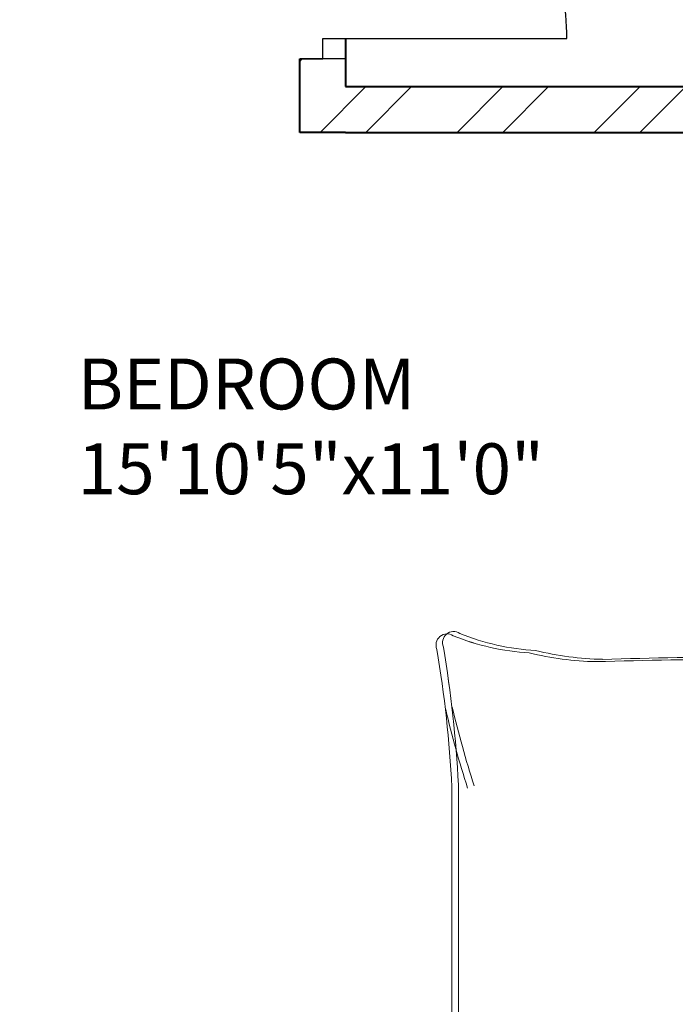
# Model space of a CAD drawing. Units: inches. Extents: x 1601 to 2297, y 1496 to 2631.
# Tile 47 of 57: x 2102 to 2167, y 2141 to 2237. Entities that reach past the tile are written whole.
import ezdxf

# ---------------------------------------------------------------- set-up
doc = ezdxf.new("R2010")
doc.units = ezdxf.units.IN
for name, color, linetype, lineweight in [('A-AREA-IDEN', 7, 'Continuous', 18), ('A-DOOR', 21, 'Continuous', 25), ('A-FURN', 8, 'Continuous', 18), ('A-WALL', 7, 'Continuous', 40), ('A-WALL-PATT', 215, 'Continuous', 13)]:
    doc.layers.add(name, color=color, linetype=linetype, lineweight=lineweight)
doc.styles.get("Standard").update_dxf_attribs({"font": 'arial.ttf'})

# ---------------------------------------------------------------- blocks, each defined once
blk = doc.blocks.new('BED-DOUBLE')
for p, q in [((79.245, 15.063), (79.245, 39.677)), ((79.245, 15.063), (79.245, 39.677)), ((79.245, 15.063), (79.245, 39.677)), ((79.245, 15.063), (79.245, 39.677)), ((79.884, 15.292), (79.884, 39.905)), ((79.884, 15.291), (79.884, 39.905)), ((79.884, 15.292), (79.884, 39.905)), ((79.884, 15.291), (79.884, 39.905))]:
    blk.add_line(p, q)
for centre, radius, start, end in [((-23.712, -17.222), 106.459, 13.38322, 17.70533), ((-23.712, -17.222), 106.459, 13.38322, 17.70533), ((-23.712, -17.222), 106.459, 13.38322, 17.70533), ((-23.712, -17.222), 106.459, 13.38322, 17.70533), ((-23.073, -16.994), 106.459, 13.38322, 17.70533), ((-23.073, -16.994), 106.459, 13.38322, 17.70533), ((-23.073, -16.994), 106.459, 13.38322, 17.70533), ((-23.073, -16.994), 106.459, 13.38322, 17.70533), ((200.837, 21.427), 121.759, 182.99578, 189.40907), ((200.837, 21.426), 121.759, 182.99578, 189.40907), ((200.837, 21.427), 121.759, 182.99578, 189.40907), ((200.837, 21.426), 121.759, 182.99578, 189.40907), ((201.476, 21.655), 121.759, 182.99578, 189.40907), ((201.476, 21.655), 121.759, 182.99578, 189.40907), ((201.476, 21.655), 121.759, 182.99578, 189.40907), ((201.476, 21.655), 121.759, 182.99578, 189.40907), ((51.253, 485.051), 482.31, 268.22771, 271.71854), ((51.253, 485.05), 482.31, 268.22771, 271.71854), ((51.253, 485.051), 482.31, 268.22771, 271.71854), ((51.253, 485.05), 482.31, 268.22771, 271.71854), ((65.154, -26.671), 29.634, 76.06484, 88.91125), ((65.154, -26.672), 29.634, 76.06484, 88.91125), ((65.154, -26.671), 29.634, 76.06484, 88.91125), ((65.154, -26.672), 29.634, 76.06484, 88.91125), ((50.614, 484.822), 482.31, 268.22771, 271.71854), ((50.614, 484.822), 482.31, 268.22771, 271.71854), ((50.614, 484.822), 482.31, 268.22771, 271.71854), ((50.614, 484.822), 482.31, 268.22771, 271.71854), ((64.515, -26.9), 29.634, 76.06484, 88.91125), ((64.515, -26.9), 29.634, 76.06484, 88.91125), ((64.515, -26.9), 29.634, 76.06484, 88.91125), ((64.515, -26.9), 29.634, 76.06484, 88.91125), ((70.915, -21.431), 23.562, 67.97508, 86.652), ((70.915, -21.432), 23.562, 67.97508, 86.652), ((70.915, -21.431), 23.562, 67.97508, 86.652), ((70.915, -21.432), 23.562, 67.97508, 86.652), ((70.276, -21.66), 23.562, 67.97508, 86.652), ((70.276, -21.66), 23.562, 67.97508, 86.652), ((70.276, -21.66), 23.562, 67.97508, 86.652), ((70.276, -21.66), 23.562, 67.97508, 86.652), ((79.718, 1.087), 1.089, 236.17358, 23.47814), ((79.718, 1.087), 1.089, 236.17358, 23.47814), ((79.718, 1.087), 1.089, 236.17358, 23.47814), ((79.718, 1.087), 1.089, 236.17358, 23.47814), ((80.357, 1.316), 1.089, 236.17358, 23.47814), ((80.357, 1.316), 1.089, 236.17358, 23.47814), ((80.357, 1.315), 1.089, 236.17358, 23.47814), ((80.357, 1.315), 1.089, 236.17358, 23.47814)]:
    blk.add_arc(centre, radius, start, end)

msp = doc.modelspace()

# ---------------------------------------------------------------- hatches: boundary and pattern name
at = {"layer": 'A-WALL-PATT'}
h = msp.add_hatch(dxfattribs=at)
h.set_pattern_fill('ANSI32', color=256)
h.paths.add_polyline_path([(1842.0336, 2528.0767), (1842.0336, 2532.3254), (1686.0373, 2532.3254), (1686.0373, 2492.9493), (1695.0373, 2492.9493), (1695.0373, 2523.3254), (1827.0373, 2523.3254), (1827.0373, 2416.8254), (1834.6225, 2416.8254), (1834.6225, 2419.0754), (1834.6225, 2421.3254), (1831.5373, 2421.3254), (1831.5373, 2523.3254), (1842.0336, 2523.3254)])
h.paths.add_polyline_path([(1695.0373, 2432.9493), (1686.0373, 2432.9493), (1686.0373, 2325.989), (1695.0373, 2325.989), (1695.0373, 2347.8254), (1827.0373, 2347.8254), (1827.0373, 2287.8254), (1823.2991, 2287.8254), (1823.2991, 2283.3254), (1847.9422, 2283.3254), (1847.9422, 2285.5754), (1847.9422, 2287.8254), (1831.5373, 2287.8254), (1831.5373, 2347.8254), (1846.9946, 2347.8254), (1846.9946, 2350.0754), (1846.9946, 2352.3254), (1695.0373, 2352.3254)])
h.paths.add_polyline_path([(1807.1169, 1573.5395), (2055.0405, 1573.5395), (2055.0405, 1610.6322), (1807.1169, 1610.6322)], flags=9)
h.paths.add_polyline_path([(1841.1631, 1712.7967), (1870.3957, 1712.7967), (1870.3957, 1731.454), (1841.1631, 1731.454)], flags=9)
h.paths.add_polyline_path([(2144.3862, 1772.185), (2191.0233, 1772.185), (2191.0233, 1790.8423), (2144.3862, 1790.8423)], flags=9)
h.paths.add_polyline_path([(2143.0128, 1827.3312), (2177.9958, 1827.3312), (2177.9958, 1845.9886), (2143.0128, 1845.9886)], flags=9)
h.paths.add_polyline_path([(2041.2439, 1833.5691), (2070.8516, 1833.5691), (2070.8516, 1852.2264), (2041.2439, 1852.2264)], flags=9)
h.paths.add_polyline_path([(2097.2791, 1947.0598), (2134.2061, 1947.0598), (2134.2061, 1965.7171), (2097.2791, 1965.7171)], flags=9)
h.paths.add_polyline_path([(2214.995, 1904.3124), (2214.995, 1942.2899), (2196.3376, 1942.2899), (2196.3376, 1904.3124)], flags=9)
h.paths.add_polyline_path([(2186.6284, 2043.8031), (2219.7935, 2043.8031), (2219.7935, 2062.4605), (2186.6284, 2062.4605)], flags=9)
h.paths.add_polyline_path([(2064.0877, 2031.616), (2097.4949, 2031.616), (2097.4949, 2050.2734), (2064.0877, 2050.2734)], flags=9)
h.paths.add_polyline_path([(1973.1349, 1986.0688), (2008.4009, 1986.0688), (2008.4009, 2004.7261), (1973.1349, 2004.7261)], flags=9)
h.paths.add_polyline_path([(1976.3676, 2106.9635), (2005.7469, 2106.9635), (2005.7469, 2125.6209), (1976.3676, 2125.6209)], flags=9)
h.paths.add_polyline_path([(1991.7852, 2180.4863), (2027.0513, 2180.4863), (2027.0513, 2199.1437), (1991.7852, 2199.1437)], flags=9)
h.paths.add_polyline_path([(2106.1801, 2187.9359), (2152.2101, 2187.9359), (2152.2101, 2206.5932), (2106.1801, 2206.5932)], flags=9)
h.paths.add_polyline_path([(2148.6686, 2262.2542), (2182.318, 2262.2542), (2182.318, 2280.9115), (2148.6686, 2280.9115)], flags=9)
h.paths.add_polyline_path([(2041.6327, 2252.8147), (2071.2405, 2252.8147), (2071.2405, 2271.4721), (2041.6327, 2271.4721)], flags=9)
h.paths.add_polyline_path([(2063.9734, 2375.4265), (2100.9004, 2375.4265), (2100.9004, 2394.0839), (2063.9734, 2394.0839)], flags=9)
h.paths.add_polyline_path([(2216.4955, 2330.9748), (2216.4955, 2370.2654), (2197.8381, 2370.2654), (2197.8381, 2330.9748)], flags=9)
h.paths.add_polyline_path([(2179.1416, 2485.8687), (2212.3067, 2485.8687), (2212.3067, 2504.5261), (2179.1416, 2504.5261)], flags=9)
h.paths.add_polyline_path([(2078.7442, 2471.1516), (2112.1514, 2471.1516), (2112.1514, 2489.809), (2078.7442, 2489.809)], flags=9)
h.paths.add_polyline_path([(1915.9631, 2329.4668), (1952.8902, 2329.4668), (1952.8902, 2348.1241), (1915.9631, 2348.1241)], flags=9)
h.paths.add_polyline_path([(1904.3189, 2499.6709), (1940.4512, 2499.6709), (1940.4512, 2518.3282), (1904.3189, 2518.3282)], flags=9)
h.paths.add_polyline_path([(1892.3665, 2100.4595), (1925.6374, 2100.4595), (1925.6374, 2119.1169), (1892.3665, 2119.1169)], flags=9)
h.paths.add_polyline_path([(1909.2984, 1805.9631), (1946.2254, 1805.9631), (1946.2254, 1824.6205), (1909.2984, 1824.6205)], flags=9)
h.paths.add_polyline_path([(1934.6056, 1658.616), (1970.738, 1658.616), (1970.738, 1677.2733), (1934.6056, 1677.2733)], flags=9)
h.paths.add_polyline_path([(1711.2052, 1789.8902), (1750.0456, 1789.8902), (1750.0456, 1808.5476), (1711.2052, 1808.5476)], flags=9)
h.paths.add_polyline_path([(1742.7874, 1854.6743), (1771.9449, 1854.6743), (1771.9449, 1873.3317), (1742.7874, 1873.3317)], flags=9)
h.paths.add_polyline_path([(1807.3592, 1997.7912), (1850.1116, 1997.7912), (1850.1116, 2016.4486), (1807.3592, 2016.4486)], flags=9)
h.paths.add_polyline_path([(1717.4579, 2237.7844), (1760.2103, 2237.7844), (1760.2103, 2256.4417), (1717.4579, 2256.4417)], flags=9)
h.paths.add_polyline_path([(1780.9285, 2324.0623), (1810.086, 2324.0623), (1810.086, 2342.7197), (1780.9285, 2342.7197)], flags=25)
h.paths.add_polyline_path([(1837.696, 2449.2024), (1866.9286, 2449.2024), (1866.9286, 2467.8598), (1837.696, 2467.8598)], flags=9)
h.paths.add_polyline_path([(1712.7752, 2484.9404), (1751.6156, 2484.9404), (1751.6156, 2503.5977), (1712.7752, 2503.5977)], flags=25)
h = msp.add_hatch(dxfattribs=at)
h.set_pattern_fill('ANSI32', color=256)
h.paths.add_polyline_path([(1973.9371, 2211.3254), (1893.0373, 2211.3254), (1893.0373, 2287.8254), (1884.6167, 2287.8254), (1884.6167, 2285.5754), (1884.6167, 2283.3254), (1888.5373, 2283.3254), (1888.5373, 2145.3254), (1695.0373, 2145.3254), (1695.0373, 2173.8724), (1690.5373, 2173.8724), (1686.0373, 2173.8724), (1686.0373, 2136.3254), (1722.5687, 2136.3254), (1722.5687, 2117.4352), (1731.5687, 2117.4352), (1731.5687, 2136.3254), (1893.0373, 2136.3254), (1893.0373, 2202.3254), (1959.0373, 2202.3254), (1959.0373, 2182.1303), (1968.0373, 2182.1303), (1968.0373, 2202.3254), (1973.9371, 2202.3254)])
h.paths.add_polyline_path([(2094.0373, 2274.6364), (2096.4294, 2274.6364), (2096.4294, 2276.8864), (2096.4294, 2279.1364), (2094.0373, 2279.1364), (2094.0373, 2290.8254), (2094.0373, 2295.3254), (2089.5373, 2295.3254), (2089.5373, 2230.8254), (2035.5373, 2230.8254), (2035.5373, 2299.8254), (2031.0373, 2299.8254), (2031.0373, 2211.3254), (2023.0065, 2211.3254), (2023.0065, 2202.3254), (2031.0373, 2202.3254), (2031.0373, 2140.8254), (1968.0373, 2140.8254), (1968.0373, 2145.9106), (1963.5373, 2145.9106), (1959.0373, 2145.9106), (1959.0373, 2116.839), (1963.5373, 2116.839), (1968.0373, 2116.839), (1968.0373, 2131.8254), (2031.0373, 2131.8254), (2031.0373, 2094.3254), (2031.0373, 2085.3254), (2031.0373, 2056.8254), (1968.0373, 2056.8254), (1968.0373, 2070.4947), (1963.5373, 2070.4947), (1959.0373, 2070.4947), (1959.0373, 2040.3029), (1968.0373, 2040.3029), (1968.0373, 2047.8254), (2031.0373, 2047.8254), (2031.0373, 1983.3254), (2031.0373, 1978.8254), (2021.1979, 1978.8254), (2021.1979, 1974.3254), (2031.0373, 1974.3254), (2031.0373, 1954.3528), (2035.5373, 1954.3528), (2035.5373, 1974.3254), (2035.5373, 1981.8254), (2055.5513, 1981.8254), (2055.5513, 1986.3254), (2035.5373, 1986.3254), (2035.5373, 2047.8254), (2040.0373, 2047.8254), (2040.0373, 2085.3254), (2040.0373, 2094.3254), (2040.0373, 2140.8254), (2035.5373, 2140.8254), (2035.5373, 2226.3254), (2089.5373, 2226.3254), (2094.0373, 2226.3254)])
h.paths.add_polyline_path([(2226.0373, 2230.8254), (2134.5373, 2230.8254), (2134.5373, 2233.5437), (2130.0373, 2233.5437), (2130.0373, 2226.3254), (2134.5373, 2226.3254), (2226.0373, 2226.3254)])
h.paths.add_polyline_path([(1807.1169, 1573.5395), (2055.0405, 1573.5395), (2055.0405, 1610.6322), (1807.1169, 1610.6322)], flags=9)
h.paths.add_polyline_path([(1841.1631, 1712.7967), (1870.3957, 1712.7967), (1870.3957, 1731.454), (1841.1631, 1731.454)], flags=9)
h.paths.add_polyline_path([(2144.3862, 1772.185), (2191.0233, 1772.185), (2191.0233, 1790.8423), (2144.3862, 1790.8423)], flags=9)
h.paths.add_polyline_path([(2143.0128, 1827.3312), (2177.9958, 1827.3312), (2177.9958, 1845.9886), (2143.0128, 1845.9886)], flags=9)
h.paths.add_polyline_path([(2041.2439, 1833.5691), (2070.8516, 1833.5691), (2070.8516, 1852.2264), (2041.2439, 1852.2264)], flags=9)
h.paths.add_polyline_path([(2097.2791, 1947.0598), (2134.2061, 1947.0598), (2134.2061, 1965.7171), (2097.2791, 1965.7171)], flags=9)
h.paths.add_polyline_path([(2214.995, 1904.3124), (2214.995, 1942.2899), (2196.3376, 1942.2899), (2196.3376, 1904.3124)], flags=9)
h.paths.add_polyline_path([(2186.6284, 2043.8031), (2219.7935, 2043.8031), (2219.7935, 2062.4605), (2186.6284, 2062.4605)], flags=9)
h.paths.add_polyline_path([(2064.0877, 2031.616), (2097.4949, 2031.616), (2097.4949, 2050.2734), (2064.0877, 2050.2734)], flags=9)
h.paths.add_polyline_path([(1973.1349, 1986.0688), (2008.4009, 1986.0688), (2008.4009, 2004.7261), (1973.1349, 2004.7261)], flags=25)
h.paths.add_polyline_path([(1976.3676, 2106.9635), (2005.7469, 2106.9635), (2005.7469, 2125.6209), (1976.3676, 2125.6209)], flags=25)
h.paths.add_polyline_path([(1991.7852, 2180.4863), (2027.0513, 2180.4863), (2027.0513, 2199.1437), (1991.7852, 2199.1437)], flags=25)
h.paths.add_polyline_path([(2106.1801, 2187.9359), (2152.2101, 2187.9359), (2152.2101, 2206.5932), (2106.1801, 2206.5932)], flags=9)
h.paths.add_polyline_path([(2148.6686, 2262.2542), (2182.318, 2262.2542), (2182.318, 2280.9115), (2148.6686, 2280.9115)], flags=9)
h.paths.add_polyline_path([(2041.6327, 2252.8147), (2071.2405, 2252.8147), (2071.2405, 2271.4721), (2041.6327, 2271.4721)], flags=25)
h.paths.add_polyline_path([(2063.9734, 2375.4265), (2100.9004, 2375.4265), (2100.9004, 2394.0839), (2063.9734, 2394.0839)], flags=9)
h.paths.add_polyline_path([(2216.4955, 2330.9748), (2216.4955, 2370.2654), (2197.8381, 2370.2654), (2197.8381, 2330.9748)], flags=9)
h.paths.add_polyline_path([(2179.1416, 2485.8687), (2212.3067, 2485.8687), (2212.3067, 2504.5261), (2179.1416, 2504.5261)], flags=9)
h.paths.add_polyline_path([(2078.7442, 2471.1516), (2112.1514, 2471.1516), (2112.1514, 2489.809), (2078.7442, 2489.809)], flags=9)
h.paths.add_polyline_path([(1915.9631, 2329.4668), (1952.8902, 2329.4668), (1952.8902, 2348.1241), (1915.9631, 2348.1241)], flags=9)
h.paths.add_polyline_path([(1904.3189, 2499.6709), (1940.4512, 2499.6709), (1940.4512, 2518.3282), (1904.3189, 2518.3282)], flags=9)
h.paths.add_polyline_path([(1892.3665, 2100.4595), (1925.6374, 2100.4595), (1925.6374, 2119.1169), (1892.3665, 2119.1169)], flags=9)
h.paths.add_polyline_path([(1909.2984, 1805.9631), (1946.2254, 1805.9631), (1946.2254, 1824.6205), (1909.2984, 1824.6205)], flags=9)
h.paths.add_polyline_path([(1934.6056, 1658.616), (1970.738, 1658.616), (1970.738, 1677.2733), (1934.6056, 1677.2733)], flags=9)
h.paths.add_polyline_path([(1711.2052, 1789.8902), (1750.0456, 1789.8902), (1750.0456, 1808.5476), (1711.2052, 1808.5476)], flags=9)
h.paths.add_polyline_path([(1742.7874, 1854.6743), (1771.9449, 1854.6743), (1771.9449, 1873.3317), (1742.7874, 1873.3317)], flags=9)
h.paths.add_polyline_path([(1807.3592, 1997.7912), (1850.1116, 1997.7912), (1850.1116, 2016.4486), (1807.3592, 2016.4486)], flags=9)
h.paths.add_polyline_path([(1717.4579, 2237.7844), (1760.2103, 2237.7844), (1760.2103, 2256.4417), (1717.4579, 2256.4417)], flags=25)
h.paths.add_polyline_path([(1780.9285, 2324.0623), (1810.086, 2324.0623), (1810.086, 2342.7197), (1780.9285, 2342.7197)], flags=9)
h.paths.add_polyline_path([(1837.696, 2449.2024), (1866.9286, 2449.2024), (1866.9286, 2467.8598), (1837.696, 2467.8598)], flags=9)
h.paths.add_polyline_path([(1712.7752, 2484.9404), (1751.6156, 2484.9404), (1751.6156, 2503.5977), (1712.7752, 2503.5977)], flags=9)
h = msp.add_hatch(dxfattribs=at)
h.set_pattern_fill('ANSI32', color=256)
h.paths.add_polyline_path([(2230.5373, 1861.8254), (2182.5373, 1861.8254), (2182.5373, 1885.3637), (2178.0373, 1885.3637), (2178.0373, 1861.8254), (2166.0373, 1861.8254), (2134.5373, 1861.8254), (2130.0373, 1861.8254), (2130.0373, 1841.4682), (2126.8833, 1841.4682), (2126.8833, 1836.9682), (2130.0373, 1836.9682), (2130.0373, 1822.7302), (2134.5373, 1822.7302), (2134.5373, 1857.3254), (2166.0373, 1857.3254), (2226.0373, 1857.3254), (2226.0373, 1846.1155), (2230.5373, 1846.1155)])
h.paths.add_polyline_path([(2226.0373, 1797.3254), (2134.5373, 1797.3254), (2134.5373, 1800.6636), (2132.2873, 1800.6636), (2130.0373, 1800.6636), (2130.0373, 1797.3254), (2130.0373, 1792.8254), (2167.7264, 1792.8254), (2226.0373, 1792.8254)])
h.paths.add_polyline_path([(2230.5373, 1822.1155), (2226.0373, 1822.1155), (2226.0373, 1760.8563), (2230.5373, 1760.8563)])
h.paths.add_polyline_path([(2230.5373, 1700.8563), (2226.0373, 1700.8563), (2226.0373, 1644.3254), (2140.2517, 1644.3254), (2140.2517, 1635.3254), (2230.5373, 1635.3254)])
h.paths.add_polyline_path([(2080.2517, 1639.8254), (2080.2517, 1644.3254), (2035.5373, 1644.3254), (2035.5373, 1792.8254), (2094.0373, 1792.8254), (2094.0373, 1797.3254), (2094.0373, 1836.9682), (2097.1057, 1836.9682), (2097.1057, 1839.2182), (2097.1057, 1841.4682), (2094.0373, 1841.4682), (2094.0373, 1862.2276), (2089.5373, 1862.2276), (2089.5373, 1797.3254), (2035.5373, 1797.3254), (2035.5373, 1857.3254), (2035.5373, 1885.0916), (2031.0373, 1885.0916), (2031.0373, 1710.3254), (2012.329, 1710.3254), (2012.329, 1701.3254), (2031.0373, 1701.3254), (2031.0373, 1644.3254), (2031.0373, 1635.3254), (2080.2517, 1635.3254)])
h.paths.add_polyline_path([(1836.0373, 1653.2033), (1842.6171, 1653.2033), (1842.6171, 1657.7033), (1842.6171, 1662.2033), (1831.5373, 1662.2033), (1831.5373, 1764.2033), (1835.3881, 1764.2033), (1835.3881, 1766.4533), (1835.3881, 1768.7033), (1831.5373, 1768.7033), (1827.0373, 1768.7033), (1827.0373, 1662.2033), (1827.0373, 1635.3254), (1836.0373, 1635.3254)])
h.paths.add_polyline_path([(1893.0373, 1701.3254), (1907.193, 1701.3254), (1907.193, 1705.8254), (1907.193, 1710.3254), (1893.0373, 1710.3254), (1893.0373, 1819.8254), (1882.6444, 1819.8254), (1882.6444, 1817.5754), (1882.6444, 1815.3254), (1888.5373, 1815.3254), (1888.5373, 1662.2033), (1884.0373, 1662.2033), (1866.6171, 1662.2033), (1866.6171, 1653.2033), (1882.391, 1653.2033), (1884.0373, 1653.2033), (1884.0373, 1635.3254), (1893.0373, 1635.3254)])
h.paths.add_polyline_path([(1739.3335, 1639.8254), (1739.3335, 1644.3254), (1695.0373, 1644.3254), (1695.0373, 1702.0135), (1690.5373, 1702.0135), (1686.0373, 1702.0135), (1686.0373, 1635.3254), (1739.3335, 1635.3254)])
h.paths.add_polyline_path([(1827.0373, 1644.3254), (1799.3335, 1644.3254), (1799.3335, 1635.3254), (1827.0373, 1635.3254)])
h.paths.add_polyline_path([(1695.0373, 1815.3254), (1849.2759, 1815.3254), (1849.2759, 1819.8254), (1807.5373, 1819.8254), (1807.5373, 1879.8254), (1851.1533, 1879.8254), (1851.1533, 1882.0754), (1851.1533, 1884.3254), (1799.3405, 1884.3254), (1799.3405, 1882.0754), (1799.3405, 1879.8254), (1803.0373, 1879.8254), (1803.0373, 1819.8254), (1695.0373, 1819.8254), (1695.0373, 1835.0458), (1690.5373, 1835.0458), (1686.0373, 1835.0458), (1686.0373, 1766.1753), (1695.0373, 1766.1753)])
h.paths.add_polyline_path([(1775.8157, 1884.3254), (1695.0373, 1884.3254), (1695.0373, 1912.9526), (1690.5373, 1912.9526), (1686.0373, 1912.9526), (1686.0373, 1859.0458), (1695.0373, 1859.0458), (1695.0373, 1879.8254), (1775.8157, 1879.8254)])
h.paths.add_polyline_path([(1893.0373, 2031.3254), (1731.5687, 2031.3254), (1731.5687, 2057.4352), (1722.5687, 2057.4352), (1722.5687, 2031.3254), (1686.0373, 2031.3254), (1686.0373, 1972.9526), (1695.0373, 1972.9526), (1695.0373, 2022.3254), (1888.5373, 2022.3254), (1888.5373, 1884.3254), (1883.4996, 1884.3254), (1883.4996, 1879.8254), (1893.0373, 1879.8254), (1893.0373, 1974.3254), (1976.6199, 1974.3254), (1976.6199, 1978.8254), (1968.0373, 1978.8254), (1968.0373, 1983.3254), (1968.0373, 2008.4756), (1963.5373, 2008.4756), (1959.0373, 2008.4756), (1959.0373, 1983.3254), (1893.0373, 1983.3254)])
h.paths.add_polyline_path([(2230.5373, 2140.4745), (2226.0373, 2140.4745), (2226.0373, 2094.3254), (2040.0373, 2094.3254), (2040.0373, 2085.3254), (2178.0373, 2085.3254), (2178.0373, 2065.6965), (2182.5373, 2065.6965), (2182.5373, 2085.3254), (2226.0373, 2085.3254), (2226.0373, 1986.3254), (2211.2679, 1986.3254), (2211.2679, 1981.8254), (2230.5373, 1981.8254)])
h.paths.add_polyline_path([(2187.6292, 1986.3254), (2182.5373, 1986.3254), (2182.5373, 2029.6965), (2178.0373, 2029.6965), (2178.0373, 1986.3254), (2099.05, 1986.3254), (2099.05, 1981.8254), (2178.0373, 1981.8254), (2178.0373, 1969.3637), (2182.5373, 1969.3637), (2182.5373, 1981.8254), (2187.6292, 1981.8254), (2187.6292, 1984.0754)])
h.paths.add_polyline_path([(1807.1169, 1573.5395), (2055.0405, 1573.5395), (2055.0405, 1610.6322), (1807.1169, 1610.6322)], flags=9)
h.paths.add_polyline_path([(1841.1631, 1712.7967), (1870.3957, 1712.7967), (1870.3957, 1731.454), (1841.1631, 1731.454)], flags=9)
h.paths.add_polyline_path([(2144.3862, 1772.185), (2191.0233, 1772.185), (2191.0233, 1790.8423), (2144.3862, 1790.8423)], flags=9)
h.paths.add_polyline_path([(2143.0128, 1827.3312), (2177.9958, 1827.3312), (2177.9958, 1845.9886), (2143.0128, 1845.9886)], flags=25)
h.paths.add_polyline_path([(2041.2439, 1833.5691), (2070.8516, 1833.5691), (2070.8516, 1852.2264), (2041.2439, 1852.2264)], flags=25)
h.paths.add_polyline_path([(2097.2791, 1947.0598), (2134.2061, 1947.0598), (2134.2061, 1965.7171), (2097.2791, 1965.7171)], flags=9)
h.paths.add_polyline_path([(2214.995, 1904.3124), (2214.995, 1942.2899), (2196.3376, 1942.2899), (2196.3376, 1904.3124)], flags=9)
h.paths.add_polyline_path([(2186.6284, 2043.8031), (2219.7935, 2043.8031), (2219.7935, 2062.4605), (2186.6284, 2062.4605)], flags=25)
h.paths.add_polyline_path([(2064.0877, 2031.616), (2097.4949, 2031.616), (2097.4949, 2050.2734), (2064.0877, 2050.2734)], flags=25)
h.paths.add_polyline_path([(1973.1349, 1986.0688), (2008.4009, 1986.0688), (2008.4009, 2004.7261), (1973.1349, 2004.7261)], flags=9)
h.paths.add_polyline_path([(1976.3676, 2106.9635), (2005.7469, 2106.9635), (2005.7469, 2125.6209), (1976.3676, 2125.6209)], flags=9)
h.paths.add_polyline_path([(1991.7852, 2180.4863), (2027.0513, 2180.4863), (2027.0513, 2199.1437), (1991.7852, 2199.1437)], flags=9)
h.paths.add_polyline_path([(2106.1801, 2187.9359), (2152.2101, 2187.9359), (2152.2101, 2206.5932), (2106.1801, 2206.5932)], flags=9)
h.paths.add_polyline_path([(2148.6686, 2262.2542), (2182.318, 2262.2542), (2182.318, 2280.9115), (2148.6686, 2280.9115)], flags=9)
h.paths.add_polyline_path([(2041.6327, 2252.8147), (2071.2405, 2252.8147), (2071.2405, 2271.4721), (2041.6327, 2271.4721)], flags=9)
h.paths.add_polyline_path([(2063.9734, 2375.4265), (2100.9004, 2375.4265), (2100.9004, 2394.0839), (2063.9734, 2394.0839)], flags=9)
h.paths.add_polyline_path([(2216.4955, 2330.9748), (2216.4955, 2370.2654), (2197.8381, 2370.2654), (2197.8381, 2330.9748)], flags=9)
h.paths.add_polyline_path([(2179.1416, 2485.8687), (2212.3067, 2485.8687), (2212.3067, 2504.5261), (2179.1416, 2504.5261)], flags=9)
h.paths.add_polyline_path([(2078.7442, 2471.1516), (2112.1514, 2471.1516), (2112.1514, 2489.809), (2078.7442, 2489.809)], flags=9)
h.paths.add_polyline_path([(1915.9631, 2329.4668), (1952.8902, 2329.4668), (1952.8902, 2348.1241), (1915.9631, 2348.1241)], flags=9)
h.paths.add_polyline_path([(1904.3189, 2499.6709), (1940.4512, 2499.6709), (1940.4512, 2518.3282), (1904.3189, 2518.3282)], flags=9)
h.paths.add_polyline_path([(1892.3665, 2100.4595), (1925.6374, 2100.4595), (1925.6374, 2119.1169), (1892.3665, 2119.1169)], flags=9)
h.paths.add_polyline_path([(1909.2984, 1805.9631), (1946.2254, 1805.9631), (1946.2254, 1824.6205), (1909.2984, 1824.6205)], flags=9)
h.paths.add_polyline_path([(1934.6056, 1658.616), (1970.738, 1658.616), (1970.738, 1677.2733), (1934.6056, 1677.2733)], flags=9)
h.paths.add_polyline_path([(1711.2052, 1789.8902), (1750.0456, 1789.8902), (1750.0456, 1808.5476), (1711.2052, 1808.5476)], flags=25)
h.paths.add_polyline_path([(1742.7874, 1854.6743), (1771.9449, 1854.6743), (1771.9449, 1873.3317), (1742.7874, 1873.3317)], flags=25)
h.paths.add_polyline_path([(1807.3592, 1997.7912), (1850.1116, 1997.7912), (1850.1116, 2016.4486), (1807.3592, 2016.4486)], flags=25)
h.paths.add_polyline_path([(1717.4579, 2237.7844), (1760.2103, 2237.7844), (1760.2103, 2256.4417), (1717.4579, 2256.4417)], flags=9)
h.paths.add_polyline_path([(1780.9285, 2324.0623), (1810.086, 2324.0623), (1810.086, 2342.7197), (1780.9285, 2342.7197)], flags=9)
h.paths.add_polyline_path([(1837.696, 2449.2024), (1866.9286, 2449.2024), (1866.9286, 2467.8598), (1837.696, 2467.8598)], flags=9)
h.paths.add_polyline_path([(1712.7752, 2484.9404), (1751.6156, 2484.9404), (1751.6156, 2503.5977), (1712.7752, 2503.5977)], flags=9)

# ---------------------------------------------------------------- linework, layer by layer
at = {"layer": 'A-DOOR'}
for p, q in [((2132.2873, 2233.5437), (2132.2873, 2235.5437)), ((2132.2873, 2235.5437), (2156.2873, 2235.5437)), ((2134.5373, 2233.5437), (2130.0373, 2233.5437)), ((2130.0373, 2233.5437), (2132.2873, 2233.5437))]:
    msp.add_line(p, q, dxfattribs=at)
msp.add_arc((2133.0674, 2235.5437), 23.2199, 360, 91.925269, dxfattribs=at)
at = {"layer": 'A-WALL'}
for p, q in [((2134.5373, 2235.5437), (2134.5373, 2230.8254)), ((2130.0373, 2226.3254), (2130.0373, 2233.5437)), ((2134.5373, 2230.8254), (2226.0373, 2230.8254)), ((2134.5373, 2226.3254), (2130.0373, 2226.3254)), ((2134.5373, 2226.3254), (2226.0373, 2226.3254))]:
    msp.add_line(p, q, dxfattribs=at)

# ---------------------------------------------------------------- block references
at = {"layer": 'A-FURN', "rotation": 180}
msp.add_blockref('BED-DOUBLE', (2224.864, 2177.2786), dxfattribs=at)

# ---------------------------------------------------------------- texts
at = {"layer": 'A-AREA-IDEN', "insert": (2108.1906, 2204.1086), "char_height": 5, "attachment_point": 1}
msp.add_mtext_dynamic_manual_height_columns('BEDROOM\\P15\'10\'5"x11\'0"', width=85.200025, gutter_width=12.5, heights=[0], dxfattribs=at)

doc.saveas('drawing.dxf')
